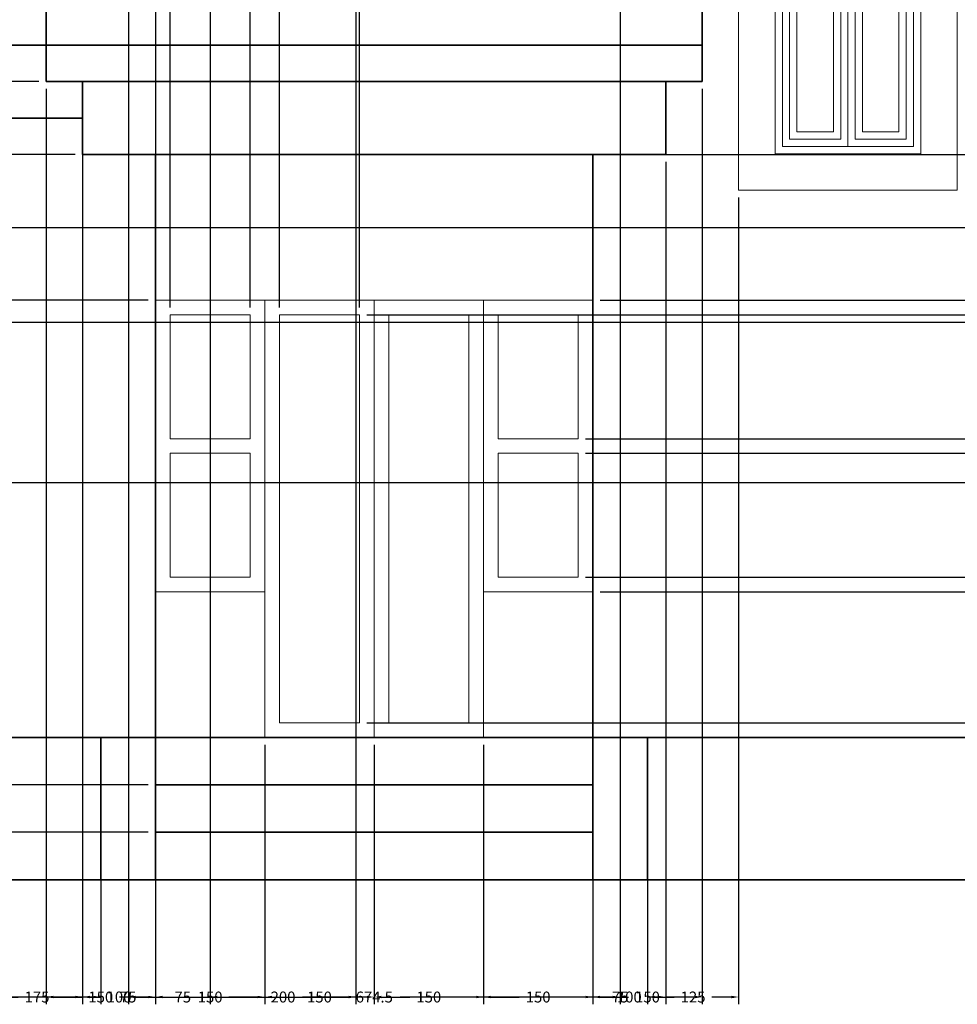
# Model space of a CAD drawing. Units: millimetres. Extents: x 937 to 4561, y 2711 to 5748.
# Tile 5 of 8: x 2543 to 3829, y 2711 to 4062. Entities that reach past the tile are written whole.
import ezdxf

# ---------------------------------------------------------------- set-up
doc = ezdxf.new("R2010")
doc.units = ezdxf.units.MM
doc.header["$MEASUREMENT"] = 0
for name, color, linetype, lineweight in [('A-ANNO-DIMS', 2, 'Continuous', 18), ('A-DOOR', 3, 'Continuous', 18), ('A-ELEV', 7, 'Continuous', 35), ('A-GLAZ', 4, 'Continuous', 18)]:
    doc.layers.add(name, color=color, linetype=linetype, lineweight=lineweight)
doc.styles.get("Standard").update_dxf_attribs({"font": 'arial.ttf'})
doc.dimstyles.get("Standard").update_dxf_attribs({"dimtxt": 15, "dimasz": 10, "dimexe": 10, "dimexo": 10, "dimgap": 10, "dimtad": 0, "dimtih": 1, "dimtoh": 1, "dimdec": 0, "dimzin": 0, "dimdsep": 46, "dimtxsty": 'Standard', "dimcen": 5, "dimadec": 0, "dimazin": 0, "dimtfac": 1, "dimtdec": 0, "dimtofl": 0, "dimtmove": 0, "dimatfit": 3, "dimfxl": 1, "dimtolj": 1, "dimtzin": 0, "dimarcsym": 0})

# ---------------------------------------------------------------- blocks, each defined once
blk = doc.blocks.new('WIN-SIDE')
for p, q in [((3529.5, 5026.9), (3529.5, 4626.9)), ((3579.5, 5026.9), (3779.5, 5026.9)), ((3579.5, 4676.9), (3579.5, 5026.9)), ((3779.5, 5026.9), (3779.5, 4676.9)), ((3829.5, 4626.9), (3829.5, 5026.9)), ((3779.5, 4676.9), (3579.5, 4676.9)), ((3529.5, 4626.9), (3829.5, 4626.9))]:
    blk.add_line(p, q)
for points in [[(3589.5, 5016.9), (3679.5, 5016.9), (3679.5, 4926.9), (3589.5, 4926.9)], [(3679.5, 5016.9), (3769.5, 5016.9), (3769.5, 4926.9), (3679.5, 4926.9)], [(3599.5, 5006.9), (3669.5, 5006.9), (3669.5, 4936.9), (3599.5, 4936.9)], [(3689.5, 5006.9), (3759.5, 5006.9), (3759.5, 4936.9), (3689.5, 4936.9)], [(3609.5, 4996.9), (3659.5, 4996.9), (3659.5, 4946.9), (3609.5, 4946.9)], [(3699.5, 4996.9), (3749.5, 4996.9), (3749.5, 4946.9), (3699.5, 4946.9)], [(3589.5, 4916.9), (3679.5, 4916.9), (3679.5, 4686.9), (3589.5, 4686.9)], [(3599.5, 4906.9), (3669.5, 4906.9), (3669.5, 4696.9), (3599.5, 4696.9)], [(3679.5, 4916.9), (3769.5, 4916.9), (3769.5, 4686.9), (3679.5, 4686.9)], [(3689.5, 4906.9), (3759.5, 4906.9), (3759.5, 4696.9), (3689.5, 4696.9)], [(3609.5, 4896.9), (3659.5, 4896.9), (3659.5, 4706.9), (3609.5, 4706.9)], [(3699.5, 4896.9), (3749.5, 4896.9), (3749.5, 4706.9), (3699.5, 4706.9)]]:
    blk.add_lwpolyline(points, close=True)
blk = doc.blocks.new('*D6')
at = {"layer": 'A-ANNO-DIMS', "color": 0, "lineweight": -2, "transparency": 16777216}
for p, q in [((2479.5, 3066.9), (2479.5, 2710.9)), ((2654.5, 3066.9), (2654.5, 2710.9)), ((2489.5, 2720.9), (2541.1, 2720.9)), ((2644.5, 2720.9), (2592.9, 2720.9))]:
    blk.add_line(p, q, dxfattribs=at)
at = {"layer": 'A-ANNO-DIMS', "color": 0, "transparency": 16777216}
for points in [[(2489.5, 2722.6), (2489.5, 2719.2), (2479.5, 2720.9)], [(2644.5, 2722.6), (2644.5, 2719.2), (2654.5, 2720.9)]]:
    blk.add_solid(points, dxfattribs=at)
at = {"layer": 'Defpoints', "color": 0, "transparency": 16777216}
for p in [(2479.5, 3076.9), (2654.5, 3076.9), (2654.5, 2720.9)]:
    blk.add_point(p, dxfattribs=at)
at = {"layer": 'A-ANNO-DIMS', "color": 0, "transparency": 16777216, "insert": (2567, 2720.9), "char_height": 15, "attachment_point": 5}
blk.add_mtext('\\A1;175', dxfattribs=at)
blk = doc.blocks.new('*D7')
at = {"layer": 'A-ANNO-DIMS', "color": 0, "lineweight": -2, "transparency": 16777216}
for p, q in [((2654.5, 3066.9), (2654.5, 2710.9)), ((2729.5, 3066.9), (2729.5, 2710.9)), ((2644.5, 2720.9), (2634.5, 2720.9)), ((2739.5, 2720.9), (2749.5, 2720.9))]:
    blk.add_line(p, q, dxfattribs=at)
at = {"layer": 'A-ANNO-DIMS', "color": 0, "transparency": 16777216}
for points in [[(2644.5, 2722.6), (2644.5, 2719.2), (2654.5, 2720.9)], [(2739.5, 2722.6), (2739.5, 2719.2), (2729.5, 2720.9)]]:
    blk.add_solid(points, dxfattribs=at)
at = {"layer": 'Defpoints', "color": 0, "transparency": 16777216}
for p in [(2654.5, 3076.9), (2729.5, 3076.9), (2729.5, 2720.9)]:
    blk.add_point(p, dxfattribs=at)
at = {"layer": 'A-ANNO-DIMS', "color": 0, "transparency": 16777216, "insert": (2692, 2720.9), "char_height": 15, "attachment_point": 5}
blk.add_mtext('\\A1;75', dxfattribs=at)
blk = doc.blocks.new('*D8')
at = {"layer": 'A-ANNO-DIMS', "color": 0, "lineweight": -2, "transparency": 16777216}
for p, q in [((2729.5, 3066.9), (2729.5, 2710.9)), ((2879.5, 3066.9), (2879.5, 2710.9)), ((2739.5, 2720.9), (2778.6, 2720.9)), ((2869.5, 2720.9), (2830.3, 2720.9))]:
    blk.add_line(p, q, dxfattribs=at)
at = {"layer": 'A-ANNO-DIMS', "color": 0, "transparency": 16777216}
for points in [[(2739.5, 2722.6), (2739.5, 2719.2), (2729.5, 2720.9)], [(2869.5, 2722.6), (2869.5, 2719.2), (2879.5, 2720.9)]]:
    blk.add_solid(points, dxfattribs=at)
at = {"layer": 'Defpoints', "color": 0, "transparency": 16777216}
for p in [(2729.5, 3076.9), (2879.5, 3076.9), (2879.5, 2720.9)]:
    blk.add_point(p, dxfattribs=at)
at = {"layer": 'A-ANNO-DIMS', "color": 0, "transparency": 16777216, "insert": (2804.5, 2720.9), "char_height": 15, "attachment_point": 5}
blk.add_mtext('\\A1;150', dxfattribs=at)
blk = doc.blocks.new('*D9')
at = {"layer": 'A-ANNO-DIMS', "color": 0, "lineweight": -2, "transparency": 16777216}
for p, q in [((2879.5, 3066.9), (2879.5, 2710.9)), ((3029.5, 3066.9), (3029.5, 2710.9)), ((2889.5, 2720.9), (2928.6, 2720.9)), ((3019.5, 2720.9), (2980.3, 2720.9))]:
    blk.add_line(p, q, dxfattribs=at)
at = {"layer": 'A-ANNO-DIMS', "color": 0, "transparency": 16777216}
for points in [[(2889.5, 2722.6), (2889.5, 2719.2), (2879.5, 2720.9)], [(3019.5, 2722.6), (3019.5, 2719.2), (3029.5, 2720.9)]]:
    blk.add_solid(points, dxfattribs=at)
at = {"layer": 'Defpoints', "color": 0, "transparency": 16777216}
for p in [(2879.5, 3076.9), (3029.5, 3076.9), (3029.5, 2720.9)]:
    blk.add_point(p, dxfattribs=at)
at = {"layer": 'A-ANNO-DIMS', "color": 0, "transparency": 16777216, "insert": (2954.5, 2720.9), "char_height": 15, "attachment_point": 5}
blk.add_mtext('\\A1;150', dxfattribs=at)
blk = doc.blocks.new('*D10')
at = {"layer": 'A-ANNO-DIMS', "color": 0, "lineweight": -2, "transparency": 16777216}
for p, q in [((3029.5, 3066.9), (3029.5, 2710.9)), ((3179.5, 3066.9), (3179.5, 2710.9)), ((3039.5, 2720.9), (3078.6, 2720.9)), ((3169.5, 2720.9), (3130.3, 2720.9))]:
    blk.add_line(p, q, dxfattribs=at)
at = {"layer": 'A-ANNO-DIMS', "color": 0, "transparency": 16777216}
for points in [[(3039.5, 2722.6), (3039.5, 2719.2), (3029.5, 2720.9)], [(3169.5, 2722.6), (3169.5, 2719.2), (3179.5, 2720.9)]]:
    blk.add_solid(points, dxfattribs=at)
at = {"layer": 'Defpoints', "color": 0, "transparency": 16777216}
for p in [(3029.5, 3076.9), (3179.5, 3076.9), (3179.5, 2720.9)]:
    blk.add_point(p, dxfattribs=at)
at = {"layer": 'A-ANNO-DIMS', "color": 0, "transparency": 16777216, "insert": (3104.5, 2720.9), "char_height": 15, "attachment_point": 5}
blk.add_mtext('\\A1;150', dxfattribs=at)
blk = doc.blocks.new('*D11')
at = {"layer": 'A-ANNO-DIMS', "color": 0, "lineweight": -2, "transparency": 16777216}
for p, q in [((3179.5, 3066.9), (3179.5, 2710.9)), ((3329.5, 3066.9), (3329.5, 2710.9)), ((3189.5, 2720.9), (3228.6, 2720.9)), ((3319.5, 2720.9), (3280.3, 2720.9))]:
    blk.add_line(p, q, dxfattribs=at)
at = {"layer": 'A-ANNO-DIMS', "color": 0, "transparency": 16777216}
for points in [[(3189.5, 2722.6), (3189.5, 2719.2), (3179.5, 2720.9)], [(3319.5, 2722.6), (3319.5, 2719.2), (3329.5, 2720.9)]]:
    blk.add_solid(points, dxfattribs=at)
at = {"layer": 'Defpoints', "color": 0, "transparency": 16777216}
for p in [(3179.5, 3076.9), (3329.5, 3076.9), (3329.5, 2720.9)]:
    blk.add_point(p, dxfattribs=at)
at = {"layer": 'A-ANNO-DIMS', "color": 0, "transparency": 16777216, "insert": (3254.5, 2720.9), "char_height": 15, "attachment_point": 5}
blk.add_mtext('\\A1;150', dxfattribs=at)
blk = doc.blocks.new('*D12')
at = {"layer": 'A-ANNO-DIMS', "color": 0, "lineweight": -2, "transparency": 16777216}
for p, q in [((3329.5, 3066.9), (3329.5, 2710.9)), ((3404.5, 3066.9), (3404.5, 2710.9)), ((3319.5, 2720.9), (3309.5, 2720.9)), ((3414.5, 2720.9), (3424.5, 2720.9))]:
    blk.add_line(p, q, dxfattribs=at)
at = {"layer": 'A-ANNO-DIMS', "color": 0, "transparency": 16777216}
for points in [[(3319.5, 2722.6), (3319.5, 2719.2), (3329.5, 2720.9)], [(3414.5, 2722.6), (3414.5, 2719.2), (3404.5, 2720.9)]]:
    blk.add_solid(points, dxfattribs=at)
at = {"layer": 'Defpoints', "color": 0, "transparency": 16777216}
for p in [(3329.5, 3076.9), (3404.5, 3076.9), (3404.5, 2720.9)]:
    blk.add_point(p, dxfattribs=at)
at = {"layer": 'A-ANNO-DIMS', "color": 0, "transparency": 16777216, "insert": (3367, 2720.9), "char_height": 15, "attachment_point": 5}
blk.add_mtext('\\A1;75', dxfattribs=at)
blk = doc.blocks.new('*D13')
at = {"layer": 'A-ANNO-DIMS', "color": 0, "lineweight": -2, "transparency": 16777216}
for p, q in [((3529.5, 3817.9), (3529.5, 2710.9)), ((3404.5, 3066.9), (3404.5, 2710.9)), ((3414.5, 2720.9), (3441.1, 2720.9)), ((3519.5, 2720.9), (3492.9, 2720.9))]:
    blk.add_line(p, q, dxfattribs=at)
at = {"layer": 'A-ANNO-DIMS', "color": 0, "transparency": 16777216}
for points in [[(3414.5, 2722.6), (3414.5, 2719.2), (3404.5, 2720.9)], [(3519.5, 2722.6), (3519.5, 2719.2), (3529.5, 2720.9)]]:
    blk.add_solid(points, dxfattribs=at)
at = {"layer": 'Defpoints', "color": 0, "transparency": 16777216}
for p in [(3529.5, 3827.9), (3404.5, 3076.9), (3529.5, 2720.9)]:
    blk.add_point(p, dxfattribs=at)
at = {"layer": 'A-ANNO-DIMS', "color": 0, "transparency": 16777216, "insert": (3467, 2720.9), "char_height": 15, "attachment_point": 5}
blk.add_mtext('\\A1;125', dxfattribs=at)
blk = doc.blocks.new('*D24')
at = {"layer": 'A-ANNO-DIMS', "color": 0, "lineweight": -2, "transparency": 16777216}
for p, q in [((2692.4, 4642.9), (2692.4, 2710.9)), ((3366.9, 4642.9), (3366.9, 2710.9)), ((2702.4, 2720.9), (2994.3, 2720.9)), ((3356.9, 2720.9), (3065.1, 2720.9))]:
    blk.add_line(p, q, dxfattribs=at)
at = {"layer": 'A-ANNO-DIMS', "color": 0, "transparency": 16777216}
for points in [[(2702.4, 2722.6), (2702.4, 2719.2), (2692.4, 2720.9)], [(3356.9, 2722.6), (3356.9, 2719.2), (3366.9, 2720.9)]]:
    blk.add_solid(points, dxfattribs=at)
at = {"layer": 'Defpoints', "color": 0, "transparency": 16777216}
for p in [(2692.4, 4652.9), (3366.9, 4652.9), (3366.9, 2720.9)]:
    blk.add_point(p, dxfattribs=at)
at = {"layer": 'A-ANNO-DIMS', "color": 0, "transparency": 16777216, "insert": (3029.7, 2720.9), "char_height": 15, "attachment_point": 5}
blk.add_mtext('\\A1;674.5', dxfattribs=at)
blk = doc.blocks.new('*D44')
at = {"layer": 'A-ANNO-DIMS', "color": 0, "lineweight": -2, "transparency": 16777216}
for p, q in [((1379.5, 3916.9), (1379.5, 2710.9)), ((2629.5, 3916.9), (2629.5, 2710.9)), ((1389.5, 2720.9), (1972.8, 2720.9)), ((2619.5, 2720.9), (2036.2, 2720.9))]:
    blk.add_line(p, q, dxfattribs=at)
at = {"layer": 'A-ANNO-DIMS', "color": 0, "transparency": 16777216}
for points in [[(1389.5, 2722.6), (1389.5, 2719.2), (1379.5, 2720.9)], [(2619.5, 2722.6), (2619.5, 2719.2), (2629.5, 2720.9)]]:
    blk.add_solid(points, dxfattribs=at)
at = {"layer": 'Defpoints', "color": 0, "transparency": 16777216}
for p in [(1379.5, 3926.9), (2629.5, 3926.9), (2629.5, 2720.9)]:
    blk.add_point(p, dxfattribs=at)
at = {"layer": 'A-ANNO-DIMS', "color": 0, "transparency": 16777216, "insert": (2004.5, 2720.9), "char_height": 15, "attachment_point": 5}
blk.add_mtext('\\A1;1250', dxfattribs=at)
blk = doc.blocks.new('*D45')
at = {"layer": 'A-ANNO-DIMS', "color": 0, "lineweight": -2, "transparency": 16777216}
for p, q in [((2579.5, 3966.9), (2579.5, 2710.9)), ((2729.5, 3866.9), (2729.5, 2710.9)), ((2589.5, 2720.9), (2628.6, 2720.9)), ((2719.5, 2720.9), (2680.3, 2720.9))]:
    blk.add_line(p, q, dxfattribs=at)
at = {"layer": 'A-ANNO-DIMS', "color": 0, "transparency": 16777216}
for points in [[(2589.5, 2722.6), (2589.5, 2719.2), (2579.5, 2720.9)], [(2719.5, 2722.6), (2719.5, 2719.2), (2729.5, 2720.9)]]:
    blk.add_solid(points, dxfattribs=at)
at = {"layer": 'Defpoints', "color": 0, "transparency": 16777216}
for p in [(2579.5, 3976.9), (2729.5, 3876.9), (2729.5, 2720.9)]:
    blk.add_point(p, dxfattribs=at)
at = {"layer": 'A-ANNO-DIMS', "color": 0, "transparency": 16777216, "insert": (2654.5, 2720.9), "char_height": 15, "attachment_point": 5}
blk.add_mtext('\\A1;150', dxfattribs=at)
blk = doc.blocks.new('*D46')
at = {"layer": 'A-ANNO-DIMS', "color": 0, "lineweight": -2, "transparency": 16777216}
for p, q in [((2629.5, 3866.9), (2629.5, 2710.9)), ((2729.5, 3866.9), (2729.5, 2710.9)), ((2639.5, 2720.9), (2653.6, 2720.9)), ((2719.5, 2720.9), (2705.3, 2720.9))]:
    blk.add_line(p, q, dxfattribs=at)
at = {"layer": 'A-ANNO-DIMS', "color": 0, "transparency": 16777216}
for points in [[(2639.5, 2722.6), (2639.5, 2719.2), (2629.5, 2720.9)], [(2719.5, 2722.6), (2719.5, 2719.2), (2729.5, 2720.9)]]:
    blk.add_solid(points, dxfattribs=at)
at = {"layer": 'Defpoints', "color": 0, "transparency": 16777216}
for p in [(2629.5, 3876.9), (2729.5, 3876.9), (2729.5, 2720.9)]:
    blk.add_point(p, dxfattribs=at)
at = {"layer": 'A-ANNO-DIMS', "color": 0, "transparency": 16777216, "insert": (2679.5, 2720.9), "char_height": 15, "attachment_point": 5}
blk.add_mtext('\\A1;100', dxfattribs=at)
blk = doc.blocks.new('*D47')
at = {"layer": 'A-ANNO-DIMS', "color": 0, "lineweight": -2, "transparency": 16777216}
for p, q in [((3329.5, 3866.9), (3329.5, 2710.9)), ((3429.5, 3866.9), (3429.5, 2710.9)), ((3339.5, 2720.9), (3353.6, 2720.9)), ((3419.5, 2720.9), (3405.3, 2720.9))]:
    blk.add_line(p, q, dxfattribs=at)
at = {"layer": 'A-ANNO-DIMS', "color": 0, "transparency": 16777216}
for points in [[(3339.5, 2722.6), (3339.5, 2719.2), (3329.5, 2720.9)], [(3419.5, 2722.6), (3419.5, 2719.2), (3429.5, 2720.9)]]:
    blk.add_solid(points, dxfattribs=at)
at = {"layer": 'Defpoints', "color": 0, "transparency": 16777216}
for p in [(3329.5, 3876.9), (3429.5, 3876.9), (3429.5, 2720.9)]:
    blk.add_point(p, dxfattribs=at)
at = {"layer": 'A-ANNO-DIMS', "color": 0, "transparency": 16777216, "insert": (3379.5, 2720.9), "char_height": 15, "attachment_point": 5}
blk.add_mtext('\\A1;100', dxfattribs=at)
blk = doc.blocks.new('*D48')
at = {"layer": 'A-ANNO-DIMS', "color": 0, "lineweight": -2, "transparency": 16777216}
for p, q in [((3479.5, 3966.9), (3479.5, 2710.9)), ((3329.5, 3866.9), (3329.5, 2710.9)), ((3339.5, 2720.9), (3378.6, 2720.9)), ((3469.5, 2720.9), (3430.3, 2720.9))]:
    blk.add_line(p, q, dxfattribs=at)
at = {"layer": 'A-ANNO-DIMS', "color": 0, "transparency": 16777216}
for points in [[(3339.5, 2722.6), (3339.5, 2719.2), (3329.5, 2720.9)], [(3469.5, 2722.6), (3469.5, 2719.2), (3479.5, 2720.9)]]:
    blk.add_solid(points, dxfattribs=at)
at = {"layer": 'Defpoints', "color": 0, "transparency": 16777216}
for p in [(3479.5, 3976.9), (3329.5, 3876.9), (3479.5, 2720.9)]:
    blk.add_point(p, dxfattribs=at)
at = {"layer": 'A-ANNO-DIMS', "color": 0, "transparency": 16777216, "insert": (3404.5, 2720.9), "char_height": 15, "attachment_point": 5}
blk.add_mtext('\\A1;150', dxfattribs=at)
blk = doc.blocks.new('*D49')
at = {"layer": 'A-ANNO-DIMS', "color": 0, "lineweight": -2, "transparency": 16777216}
for p, q in [((2729.5, 4242.9), (2729.5, 2710.9)), ((2804.5, 4217.9), (2804.5, 2710.9)), ((2719.5, 2720.9), (2709.5, 2720.9)), ((2814.5, 2720.9), (2824.5, 2720.9))]:
    blk.add_line(p, q, dxfattribs=at)
at = {"layer": 'A-ANNO-DIMS', "color": 0, "transparency": 16777216}
for points in [[(2719.5, 2722.6), (2719.5, 2719.2), (2729.5, 2720.9)], [(2814.5, 2722.6), (2814.5, 2719.2), (2804.5, 2720.9)]]:
    blk.add_solid(points, dxfattribs=at)
at = {"layer": 'Defpoints', "color": 0, "transparency": 16777216}
for p in [(2729.5, 4252.9), (2804.5, 4227.9), (2804.5, 2720.9)]:
    blk.add_point(p, dxfattribs=at)
at = {"layer": 'A-ANNO-DIMS', "color": 0, "transparency": 16777216, "insert": (2767, 2720.9), "char_height": 15, "attachment_point": 5}
blk.add_mtext('\\A1;75', dxfattribs=at)
blk = doc.blocks.new('*D50')
at = {"layer": 'A-ANNO-DIMS', "color": 0, "lineweight": -2, "transparency": 16777216}
for p, q in [((2804.5, 4217.9), (2804.5, 2710.9)), ((3004.5, 4217.9), (3004.5, 2710.9)), ((2814.5, 2720.9), (2877.8, 2720.9)), ((2994.5, 2720.9), (2931.2, 2720.9))]:
    blk.add_line(p, q, dxfattribs=at)
at = {"layer": 'A-ANNO-DIMS', "color": 0, "transparency": 16777216}
for points in [[(2814.5, 2722.6), (2814.5, 2719.2), (2804.5, 2720.9)], [(2994.5, 2722.6), (2994.5, 2719.2), (3004.5, 2720.9)]]:
    blk.add_solid(points, dxfattribs=at)
at = {"layer": 'Defpoints', "color": 0, "transparency": 16777216}
for p in [(2804.5, 4227.9), (3004.5, 4227.9), (3004.5, 2720.9)]:
    blk.add_point(p, dxfattribs=at)
at = {"layer": 'A-ANNO-DIMS', "color": 0, "transparency": 16777216, "insert": (2904.5, 2720.9), "char_height": 15, "attachment_point": 5}
blk.add_mtext('\\A1;200', dxfattribs=at)
blk = doc.blocks.new('*D53')
at = {"layer": 'A-ANNO-DIMS', "color": 0, "lineweight": -2, "transparency": 16777216}
for p, q in [((2749.5, 3666.9), (2749.5, 5747.9)), ((2859.5, 3666.9), (2859.5, 5747.9)), ((2759.5, 5737.9), (2778.6, 5737.9)), ((2849.5, 5737.9), (2830.3, 5737.9))]:
    blk.add_line(p, q, dxfattribs=at)
at = {"layer": 'A-ANNO-DIMS', "color": 0, "transparency": 16777216}
for points in [[(2759.5, 5739.6), (2759.5, 5736.2), (2749.5, 5737.9)], [(2849.5, 5739.6), (2849.5, 5736.2), (2859.5, 5737.9)]]:
    blk.add_solid(points, dxfattribs=at)
at = {"layer": 'Defpoints', "color": 0, "transparency": 16777216}
for p in [(2859.5, 5737.9), (2749.5, 3656.9), (2859.5, 3656.9)]:
    blk.add_point(p, dxfattribs=at)
at = {"layer": 'A-ANNO-DIMS', "color": 0, "transparency": 16777216, "insert": (2804.5, 5737.9), "char_height": 15, "attachment_point": 5}
blk.add_mtext('\\A1;110', dxfattribs=at)
blk = doc.blocks.new('*D54')
at = {"layer": 'A-ANNO-DIMS', "color": 0, "lineweight": -2, "transparency": 16777216}
for p, q in [((2899.5, 3666.9), (2899.5, 5747.9)), ((3009.5, 3666.9), (3009.5, 5747.9)), ((2909.5, 5737.9), (2928.6, 5737.9)), ((2999.5, 5737.9), (2980.3, 5737.9))]:
    blk.add_line(p, q, dxfattribs=at)
at = {"layer": 'A-ANNO-DIMS', "color": 0, "transparency": 16777216}
for points in [[(2909.5, 5739.6), (2909.5, 5736.2), (2899.5, 5737.9)], [(2999.5, 5739.6), (2999.5, 5736.2), (3009.5, 5737.9)]]:
    blk.add_solid(points, dxfattribs=at)
at = {"layer": 'Defpoints', "color": 0, "transparency": 16777216}
for p in [(3009.5, 5737.9), (2899.5, 3656.9), (3009.5, 3656.9)]:
    blk.add_point(p, dxfattribs=at)
at = {"layer": 'A-ANNO-DIMS', "color": 0, "transparency": 16777216, "insert": (2954.5, 5737.9), "char_height": 15, "attachment_point": 5}
blk.add_mtext('\\A1;110', dxfattribs=at)
blk = doc.blocks.new('*D72')
at = {"layer": 'A-ANNO-DIMS', "color": 0, "lineweight": -2, "transparency": 16777216}
for p, q in [((1764.5, 3646.9), (4500.5, 3646.9)), ((4490.5, 3636.9), (4490.5, 3554.6)), ((4490.5, 3436.9), (4490.5, 3519.2)), ((1764.5, 3426.9), (4500.5, 3426.9))]:
    blk.add_line(p, q, dxfattribs=at)
at = {"layer": 'A-ANNO-DIMS', "color": 0, "transparency": 16777216}
for points in [[(4488.8, 3636.9), (4492.2, 3636.9), (4490.5, 3646.9)], [(4488.8, 3436.9), (4492.2, 3436.9), (4490.5, 3426.9)]]:
    blk.add_solid(points, dxfattribs=at)
at = {"layer": 'Defpoints', "color": 0, "transparency": 16777216}
for p in [(1754.5, 3646.9), (4490.5, 3646.9), (1754.5, 3426.9)]:
    blk.add_point(p, dxfattribs=at)
at = {"layer": 'A-ANNO-DIMS', "color": 0, "transparency": 16777216, "insert": (4490.5, 3536.9), "char_height": 15, "attachment_point": 5}
blk.add_mtext('\\A1;220', dxfattribs=at)
blk = doc.blocks.new('*D73')
at = {"layer": 'A-ANNO-DIMS', "color": 0, "lineweight": -2, "transparency": 16777216}
for p, q in [((1764.5, 3776.9), (4500.5, 3776.9)), ((4490.5, 3766.9), (4490.5, 3729.6)), ((4490.5, 3656.9), (4490.5, 3694.2)), ((1764.5, 3646.9), (4500.5, 3646.9))]:
    blk.add_line(p, q, dxfattribs=at)
at = {"layer": 'A-ANNO-DIMS', "color": 0, "transparency": 16777216}
for points in [[(4488.8, 3766.9), (4492.2, 3766.9), (4490.5, 3776.9)], [(4488.8, 3656.9), (4492.2, 3656.9), (4490.5, 3646.9)]]:
    blk.add_solid(points, dxfattribs=at)
at = {"layer": 'Defpoints', "color": 0, "transparency": 16777216}
for p in [(1754.5, 3776.9), (4490.5, 3776.9), (1754.5, 3646.9)]:
    blk.add_point(p, dxfattribs=at)
at = {"layer": 'A-ANNO-DIMS', "color": 0, "transparency": 16777216, "insert": (4490.5, 3711.9), "char_height": 15, "attachment_point": 5}
blk.add_mtext('\\A1;130', dxfattribs=at)
blk = doc.blocks.new('*D82')
at = {"layer": 'A-ANNO-DIMS', "color": 0, "lineweight": -2, "transparency": 16777216}
for p, q in [((2719.5, 3676.9), (958.5, 3676.9)), ((968.5, 3666.9), (968.5, 3394.6)), ((968.5, 3086.9), (968.5, 3359.2)), ((2719.5, 3076.9), (958.5, 3076.9))]:
    blk.add_line(p, q, dxfattribs=at)
at = {"layer": 'A-ANNO-DIMS', "color": 0, "transparency": 16777216}
for points in [[(966.8, 3666.9), (970.2, 3666.9), (968.5, 3676.9)], [(966.8, 3086.9), (970.2, 3086.9), (968.5, 3076.9)]]:
    blk.add_solid(points, dxfattribs=at)
at = {"layer": 'Defpoints', "color": 0, "transparency": 16777216}
for p in [(968.5, 3676.9), (2729.5, 3676.9), (2729.5, 3076.9)]:
    blk.add_point(p, dxfattribs=at)
at = {"layer": 'A-ANNO-DIMS', "color": 0, "transparency": 16777216, "insert": (968.5, 3376.9), "char_height": 15, "attachment_point": 5}
blk.add_mtext('\\A1;600', dxfattribs=at)
blk = doc.blocks.new('*D83')
at = {"layer": 'A-ANNO-DIMS', "color": 0, "lineweight": -2, "transparency": 16777216}
for p, q in [((2619.5, 3876.9), (958.5, 3876.9)), ((968.5, 3866.9), (968.5, 3794.6)), ((968.5, 3686.9), (968.5, 3759.2)), ((2719.5, 3676.9), (958.5, 3676.9))]:
    blk.add_line(p, q, dxfattribs=at)
at = {"layer": 'A-ANNO-DIMS', "color": 0, "transparency": 16777216}
for points in [[(966.8, 3866.9), (970.2, 3866.9), (968.5, 3876.9)], [(966.8, 3686.9), (970.2, 3686.9), (968.5, 3676.9)]]:
    blk.add_solid(points, dxfattribs=at)
at = {"layer": 'Defpoints', "color": 0, "transparency": 16777216}
for p in [(968.5, 3876.9), (2629.5, 3876.9), (2729.5, 3676.9)]:
    blk.add_point(p, dxfattribs=at)
at = {"layer": 'A-ANNO-DIMS', "color": 0, "transparency": 16777216, "insert": (968.5, 3776.9), "char_height": 15, "attachment_point": 5}
blk.add_mtext('\\A1;200', dxfattribs=at)
blk = doc.blocks.new('*D84')
at = {"layer": 'A-ANNO-DIMS', "color": 0, "lineweight": -2, "transparency": 16777216}
for p, q in [((2569.5, 3976.9), (958.5, 3976.9)), ((968.5, 3966.9), (968.5, 3944.6)), ((968.5, 3886.9), (968.5, 3909.2)), ((2619.5, 3876.9), (958.5, 3876.9))]:
    blk.add_line(p, q, dxfattribs=at)
at = {"layer": 'A-ANNO-DIMS', "color": 0, "transparency": 16777216}
for points in [[(966.8, 3966.9), (970.2, 3966.9), (968.5, 3976.9)], [(966.8, 3886.9), (970.2, 3886.9), (968.5, 3876.9)]]:
    blk.add_solid(points, dxfattribs=at)
at = {"layer": 'Defpoints', "color": 0, "transparency": 16777216}
for p in [(968.5, 3976.9), (2579.5, 3976.9), (2629.5, 3876.9)]:
    blk.add_point(p, dxfattribs=at)
at = {"layer": 'A-ANNO-DIMS', "color": 0, "transparency": 16777216, "insert": (968.5, 3926.9), "char_height": 15, "attachment_point": 5}
blk.add_mtext('\\A1;100', dxfattribs=at)
blk = doc.blocks.new('*D85')
at = {"layer": 'A-ANNO-DIMS', "color": 0, "lineweight": -2, "transparency": 16777216}
for p, q in [((2569.5, 4026.9), (958.5, 4026.9)), ((968.5, 4026.9), (968.5, 4036.9)), ((968.5, 4036.9), (978.5, 4036.9)), ((968.5, 3986.9), (968.5, 4016.9)), ((2569.5, 3976.9), (958.5, 3976.9))]:
    blk.add_line(p, q, dxfattribs=at)
at = {"layer": 'A-ANNO-DIMS', "color": 0, "transparency": 16777216}
for points in [[(966.8, 4016.9), (970.2, 4016.9), (968.5, 4026.9)], [(966.8, 3986.9), (970.2, 3986.9), (968.5, 3976.9)]]:
    blk.add_solid(points, dxfattribs=at)
at = {"layer": 'Defpoints', "color": 0, "transparency": 16777216}
for p in [(968.5, 4026.9), (2579.5, 4026.9), (2579.5, 3976.9)]:
    blk.add_point(p, dxfattribs=at)
at = {"layer": 'A-ANNO-DIMS', "color": 0, "transparency": 16777216, "insert": (999.2, 4036.9), "char_height": 15, "attachment_point": 5}
blk.add_mtext('\\A1;50', dxfattribs=at)
blk = doc.blocks.new('*D86')
at = {"layer": 'A-ANNO-DIMS', "color": 0, "lineweight": -2, "transparency": 16777216}
for p, q in [((968.5, 4076.9), (968.5, 4086.9)), ((968.5, 4086.9), (978.5, 4086.9)), ((2569.5, 4076.9), (958.5, 4076.9)), ((968.5, 4036.9), (968.5, 4066.9)), ((2569.5, 4026.9), (958.5, 4026.9))]:
    blk.add_line(p, q, dxfattribs=at)
at = {"layer": 'A-ANNO-DIMS', "color": 0, "transparency": 16777216}
for points in [[(966.8, 4066.9), (970.2, 4066.9), (968.5, 4076.9)], [(966.8, 4036.9), (970.2, 4036.9), (968.5, 4026.9)]]:
    blk.add_solid(points, dxfattribs=at)
at = {"layer": 'Defpoints', "color": 0, "transparency": 16777216}
for p in [(968.5, 4076.9), (2579.5, 4076.9), (2579.5, 4026.9)]:
    blk.add_point(p, dxfattribs=at)
at = {"layer": 'A-ANNO-DIMS', "color": 0, "transparency": 16777216, "insert": (999.2, 4086.9), "char_height": 15, "attachment_point": 5}
blk.add_mtext('\\A1;50', dxfattribs=at)
blk = doc.blocks.new('*D94')
at = {"layer": 'A-ANNO-DIMS', "color": 0, "lineweight": -2, "transparency": 16777216}
for p, q in [((3339.5, 3276.9), (4500.5, 3276.9)), ((4490.5, 3266.9), (4490.5, 3194.6)), ((4490.5, 3086.9), (4490.5, 3159.2)), ((3339.5, 3076.9), (4500.5, 3076.9))]:
    blk.add_line(p, q, dxfattribs=at)
at = {"layer": 'A-ANNO-DIMS', "color": 0, "transparency": 16777216}
for points in [[(4488.8, 3266.9), (4492.2, 3266.9), (4490.5, 3276.9)], [(4488.8, 3086.9), (4492.2, 3086.9), (4490.5, 3076.9)]]:
    blk.add_solid(points, dxfattribs=at)
at = {"layer": 'Defpoints', "color": 0, "transparency": 16777216}
for p in [(3329.5, 3276.9), (4490.5, 3276.9), (3329.5, 3076.9)]:
    blk.add_point(p, dxfattribs=at)
at = {"layer": 'A-ANNO-DIMS', "color": 0, "transparency": 16777216, "insert": (4490.5, 3176.9), "char_height": 15, "attachment_point": 5}
blk.add_mtext('\\A1;200', dxfattribs=at)
blk = doc.blocks.new('*D95')
at = {"layer": 'A-ANNO-DIMS', "color": 0, "lineweight": -2, "transparency": 16777216}
for p, q in [((3319.5, 3486.9), (4500.5, 3486.9)), ((4490.5, 3476.9), (4490.5, 3409.6)), ((4490.5, 3306.9), (4490.5, 3374.2)), ((3319.5, 3296.9), (4500.5, 3296.9))]:
    blk.add_line(p, q, dxfattribs=at)
at = {"layer": 'A-ANNO-DIMS', "color": 0, "transparency": 16777216}
for points in [[(4488.8, 3476.9), (4492.2, 3476.9), (4490.5, 3486.9)], [(4488.8, 3306.9), (4492.2, 3306.9), (4490.5, 3296.9)]]:
    blk.add_solid(points, dxfattribs=at)
at = {"layer": 'Defpoints', "color": 0, "transparency": 16777216}
for p in [(3309.5, 3486.9), (4490.5, 3486.9), (3309.5, 3296.9)]:
    blk.add_point(p, dxfattribs=at)
at = {"layer": 'A-ANNO-DIMS', "color": 0, "transparency": 16777216, "insert": (4490.5, 3391.9), "char_height": 15, "attachment_point": 5}
blk.add_mtext('\\A1;190', dxfattribs=at)
blk = doc.blocks.new('*D96')
at = {"layer": 'A-ANNO-DIMS', "color": 0, "lineweight": -2, "transparency": 16777216}
for p, q in [((3319.5, 3656.9), (4500.5, 3656.9)), ((4490.5, 3646.9), (4490.5, 3579.6)), ((4490.5, 3476.9), (4490.5, 3544.2)), ((3319.5, 3466.9), (4500.5, 3466.9))]:
    blk.add_line(p, q, dxfattribs=at)
at = {"layer": 'A-ANNO-DIMS', "color": 0, "transparency": 16777216}
for points in [[(4488.8, 3646.9), (4492.2, 3646.9), (4490.5, 3656.9)], [(4488.8, 3476.9), (4492.2, 3476.9), (4490.5, 3466.9)]]:
    blk.add_solid(points, dxfattribs=at)
at = {"layer": 'Defpoints', "color": 0, "transparency": 16777216}
for p in [(3309.5, 3656.9), (4490.5, 3656.9), (3309.5, 3466.9)]:
    blk.add_point(p, dxfattribs=at)
at = {"layer": 'A-ANNO-DIMS', "color": 0, "transparency": 16777216, "insert": (4490.5, 3561.9), "char_height": 15, "attachment_point": 5}
blk.add_mtext('\\A1;190', dxfattribs=at)
blk = doc.blocks.new('*D97')
at = {"layer": 'A-ANNO-DIMS', "color": 0, "lineweight": -2, "transparency": 16777216}
for p, q in [((3339.5, 3876.9), (4500.5, 3876.9)), ((4490.5, 3866.9), (4490.5, 3794.6)), ((4490.5, 3686.9), (4490.5, 3759.2)), ((3339.5, 3676.9), (4500.5, 3676.9))]:
    blk.add_line(p, q, dxfattribs=at)
at = {"layer": 'A-ANNO-DIMS', "color": 0, "transparency": 16777216}
for points in [[(4488.8, 3866.9), (4492.2, 3866.9), (4490.5, 3876.9)], [(4488.8, 3686.9), (4492.2, 3686.9), (4490.5, 3676.9)]]:
    blk.add_solid(points, dxfattribs=at)
at = {"layer": 'Defpoints', "color": 0, "transparency": 16777216}
for p in [(3329.5, 3876.9), (4490.5, 3876.9), (3329.5, 3676.9)]:
    blk.add_point(p, dxfattribs=at)
at = {"layer": 'A-ANNO-DIMS', "color": 0, "transparency": 16777216, "insert": (4490.5, 3776.9), "char_height": 15, "attachment_point": 5}
blk.add_mtext('\\A1;200', dxfattribs=at)
blk = doc.blocks.new('*D98')
at = {"layer": 'A-ANNO-DIMS', "color": 0, "lineweight": -2, "transparency": 16777216}
for p, q in [((3019.5, 3656.9), (4500.5, 3656.9)), ((4490.5, 3646.9), (4490.5, 3394.6)), ((4490.5, 3106.9), (4490.5, 3359.2)), ((3019.5, 3096.9), (4500.5, 3096.9))]:
    blk.add_line(p, q, dxfattribs=at)
at = {"layer": 'A-ANNO-DIMS', "color": 0, "transparency": 16777216}
for points in [[(4488.8, 3646.9), (4492.2, 3646.9), (4490.5, 3656.9)], [(4488.8, 3106.9), (4492.2, 3106.9), (4490.5, 3096.9)]]:
    blk.add_solid(points, dxfattribs=at)
at = {"layer": 'Defpoints', "color": 0, "transparency": 16777216}
for p in [(3009.5, 3656.9), (4490.5, 3656.9), (3009.5, 3096.9)]:
    blk.add_point(p, dxfattribs=at)
at = {"layer": 'A-ANNO-DIMS', "color": 0, "transparency": 16777216, "insert": (4490.5, 3376.9), "char_height": 15, "attachment_point": 5}
blk.add_mtext('\\A1;560', dxfattribs=at)
blk = doc.blocks.new('*D99')
at = {"layer": 'A-ANNO-DIMS', "color": 0, "lineweight": -2, "transparency": 16777216}
for p, q in [((2719.5, 2946.9), (958.5, 2946.9)), ((968.5, 2946.9), (968.5, 2956.9)), ((968.5, 2956.9), (978.5, 2956.9)), ((968.5, 2891.9), (968.5, 2936.9)), ((2644.5, 2881.9), (958.5, 2881.9))]:
    blk.add_line(p, q, dxfattribs=at)
at = {"layer": 'A-ANNO-DIMS', "color": 0, "transparency": 16777216}
for points in [[(966.8, 2936.9), (970.2, 2936.9), (968.5, 2946.9)], [(966.8, 2891.9), (970.2, 2891.9), (968.5, 2881.9)]]:
    blk.add_solid(points, dxfattribs=at)
at = {"layer": 'Defpoints', "color": 0, "transparency": 16777216}
for p in [(968.5, 2946.9), (2729.5, 2946.9), (2654.5, 2881.9)]:
    blk.add_point(p, dxfattribs=at)
at = {"layer": 'A-ANNO-DIMS', "color": 0, "transparency": 16777216, "insert": (999.3, 2956.9), "char_height": 15, "attachment_point": 5}
blk.add_mtext('\\A1;65', dxfattribs=at)
blk = doc.blocks.new('*D100')
at = {"layer": 'A-ANNO-DIMS', "color": 0, "lineweight": -2, "transparency": 16777216}
for p, q in [((968.5, 3011.9), (968.5, 3021.9)), ((968.5, 3021.9), (978.5, 3021.9)), ((2719.5, 3011.9), (958.5, 3011.9)), ((968.5, 2956.9), (968.5, 3001.9)), ((2719.5, 2946.9), (958.5, 2946.9))]:
    blk.add_line(p, q, dxfattribs=at)
at = {"layer": 'A-ANNO-DIMS', "color": 0, "transparency": 16777216}
for points in [[(966.8, 3001.9), (970.2, 3001.9), (968.5, 3011.9)], [(966.8, 2956.9), (970.2, 2956.9), (968.5, 2946.9)]]:
    blk.add_solid(points, dxfattribs=at)
at = {"layer": 'Defpoints', "color": 0, "transparency": 16777216}
for p in [(968.5, 3011.9), (2729.5, 3011.9), (2729.5, 2946.9)]:
    blk.add_point(p, dxfattribs=at)
at = {"layer": 'A-ANNO-DIMS', "color": 0, "transparency": 16777216, "insert": (999.3, 3021.9), "char_height": 15, "attachment_point": 5}
blk.add_mtext('\\A1;65', dxfattribs=at)
blk = doc.blocks.new('*D101')
at = {"layer": 'A-ANNO-DIMS', "color": 0, "lineweight": -2, "transparency": 16777216}
for p, q in [((968.5, 3076.9), (968.5, 3086.9)), ((968.5, 3086.9), (978.5, 3086.9)), ((2644.5, 3076.9), (958.5, 3076.9)), ((968.5, 3021.9), (968.5, 3066.9)), ((2719.5, 3011.9), (958.5, 3011.9))]:
    blk.add_line(p, q, dxfattribs=at)
at = {"layer": 'A-ANNO-DIMS', "color": 0, "transparency": 16777216}
for points in [[(966.8, 3066.9), (970.2, 3066.9), (968.5, 3076.9)], [(966.8, 3021.9), (970.2, 3021.9), (968.5, 3011.9)]]:
    blk.add_solid(points, dxfattribs=at)
at = {"layer": 'Defpoints', "color": 0, "transparency": 16777216}
for p in [(968.5, 3076.9), (2654.5, 3076.9), (2729.5, 3011.9)]:
    blk.add_point(p, dxfattribs=at)
at = {"layer": 'A-ANNO-DIMS', "color": 0, "transparency": 16777216, "insert": (999.3, 3086.9), "char_height": 15, "attachment_point": 5}
blk.add_mtext('\\A1;65', dxfattribs=at)

msp = doc.modelspace()

# ---------------------------------------------------------------- linework, layer by layer
at = {"layer": 'A-DOOR'}
for p, q in [((2879.4852, 3676.9013), (3029.4852, 3676.9013)), ((2879.4852, 3076.9013), (2879.4852, 3676.9013)), ((3029.4852, 3676.9013), (3179.4852, 3676.9013)), ((3029.4852, 3076.9013), (3029.4852, 3676.9013)), ((3029.4852, 3676.9013), (3029.4852, 3076.9013)), ((3179.4852, 3676.9013), (3179.4852, 3076.9013)), ((2899.4852, 3656.9013), (3009.4852, 3656.9013)), ((2899.4852, 3096.9013), (2899.4852, 3656.9013)), ((3009.4852, 3656.9013), (3009.4852, 3096.9013)), ((3049.4852, 3656.9013), (3159.4852, 3656.9013)), ((3049.4852, 3096.9013), (3049.4852, 3656.9013)), ((3159.4852, 3656.9013), (3159.4852, 3096.9013)), ((2749.4852, 3486.9013), (2859.4852, 3486.9013)), ((3199.4852, 3486.9013), (3309.4852, 3486.9013)), ((2749.4852, 3466.9013), (2859.4852, 3466.9013)), ((3199.4852, 3466.9013), (3309.4852, 3466.9013)), ((3009.4852, 3096.9013), (2899.4852, 3096.9013)), ((3159.4852, 3096.9013), (3049.4852, 3096.9013)), ((3029.4852, 3076.9013), (2879.4852, 3076.9013)), ((3179.4852, 3076.9013), (3029.4852, 3076.9013))]:
    msp.add_line(p, q, dxfattribs=at)
for points in [[(2729.4852, 3676.9013), (2879.4852, 3676.9013), (2879.4852, 3276.9013), (2729.4852, 3276.9013)], [(3179.4852, 3676.9013), (3329.4852, 3676.9013), (3329.4852, 3276.9013), (3179.4852, 3276.9013)]]:
    msp.add_lwpolyline(points, close=True, dxfattribs=at)
for points in [[(2749.4852, 3486.9013), (2749.4852, 3656.9013), (2859.4852, 3656.9013), (2859.4852, 3486.9013)], [(3199.4852, 3486.9013), (3199.4852, 3656.9013), (3309.4852, 3656.9013), (3309.4852, 3486.9013)], [(2859.4852, 3466.9013), (2859.4852, 3296.9013), (2749.4852, 3296.9013), (2749.4852, 3466.9013)], [(3309.4852, 3466.9013), (3309.4852, 3296.9013), (3199.4852, 3296.9013), (3199.4852, 3466.9013)]]:
    msp.add_lwpolyline(points, dxfattribs=at)
at = {"layer": 'A-ELEV'}
for p, q in [((2579.4852, 4076.9013), (2579.4852, 3976.9013)), ((3479.4852, 4076.9013), (3479.4852, 3976.9013)), ((1429.4852, 4026.9013), (3479.4852, 4026.9013)), ((2729.4852, 4026.9013), (2579.4852, 4026.9013)), ((3329.4852, 4026.9013), (3479.4852, 4026.9013)), ((2579.4852, 3976.9013), (3479.4852, 3976.9013)), ((2579.4852, 3976.9013), (2629.4852, 3976.9013)), ((2729.4852, 3976.9013), (2629.4852, 3976.9013)), ((2629.4852, 3976.9013), (2629.4852, 3876.9013)), ((3329.4852, 3976.9013), (3429.4852, 3976.9013)), ((3479.4852, 3976.9013), (3429.4852, 3976.9013)), ((3429.4852, 3976.9013), (3429.4852, 3876.9013)), ((1429.4852, 3926.9013), (2629.4852, 3926.9013)), ((2629.4852, 3876.9013), (2729.4852, 3876.9013)), ((2629.4852, 3876.9013), (2729.4852, 3876.9013)), ((2729.4852, 2881.9013), (2729.4852, 3876.9013)), ((2729.4852, 3876.9013), (3429.4852, 3876.9013)), ((3329.4852, 2881.9013), (3329.4852, 3876.9013)), ((3429.4852, 3876.9013), (3329.4852, 3876.9013)), ((1429.4852, 3076.9013), (4029.4852, 3076.9013)), ((2729.4852, 3076.9013), (2654.4852, 3076.9013)), ((2654.4852, 3076.9013), (2654.4852, 2881.9013)), ((3329.4852, 3076.9013), (3404.4852, 3076.9013)), ((3404.4852, 3076.9013), (3404.4852, 2881.9013)), ((2729.4852, 3011.9013), (3329.4852, 3011.9013)), ((2729.4852, 2946.9013), (3329.4852, 2946.9013)), ((1429.4852, 2881.9013), (4029.4852, 2881.9013))]:
    msp.add_line(p, q, dxfattribs=at)

# ---------------------------------------------------------------- block references
at = {"layer": 'A-GLAZ'}
msp.add_blockref('WIN-SIDE', (0, -799.0013), dxfattribs=at)

# ---------------------------------------------------------------- dimensions: what is measured, and where the dimension line sits
at = {"layer": 'A-ANNO-DIMS'}
for base, p1, p2, override, picture, middle in [((2859.4852, 5737.9013), (2749.4852, 3656.9013), (2859.4852, 3656.9013), {"dimdec": 0, "dimlfac": 1, "dimrnd": 0, "dimzin": 0, "dimdsep": 46, "dimlunit": 2}, '*D53', (2804.4852, 5737.9013)), ((3009.4852, 5737.9013), (2899.4852, 3656.9013), (3009.4852, 3656.9013), {"dimdec": 0, "dimlfac": 1, "dimrnd": 0, "dimzin": 0, "dimdsep": 46, "dimlunit": 2}, '*D54', (2954.4852, 5737.9013)), ((3366.9387, 2720.9013), (2692.4029, 4652.9001), (3366.9387, 4652.9001), {"dimdec": 1, "dimlfac": 1, "dimrnd": 0, "dimzin": 0, "dimdsep": 46, "dimlunit": 2}, '*D24', (3029.6708, 2720.9013)), ((2804.4852, 2720.9013), (2729.4852, 4252.9001), (2804.4852, 4227.9047), {"dimdec": 0, "dimlfac": 1, "dimrnd": 0, "dimzin": 0, "dimdsep": 46, "dimlunit": 2}, '*D49', (2766.9852, 2720.9013)), ((3004.4852, 2720.9013), (2804.4852, 4227.9047), (3004.4852, 4227.9047), {"dimdec": 0, "dimlfac": 1, "dimrnd": 0, "dimzin": 0, "dimdsep": 46, "dimlunit": 2}, '*D50', (2904.4852, 2720.9013)), ((2729.4852, 2720.9013), (2579.4852, 3976.9013), (2729.4852, 3876.9013), {"dimdec": 0, "dimlfac": 1, "dimrnd": 0, "dimzin": 0, "dimdsep": 46, "dimlunit": 2}, '*D45', (2654.4852, 2720.9013)), ((3479.4852, 2720.9013), (3329.4852, 3876.9013), (3479.4852, 3976.9013), {"dimdec": 0, "dimlfac": 1, "dimrnd": 0, "dimzin": 0, "dimdsep": 46, "dimlunit": 2}, '*D48', (3404.4852, 2720.9013)), ((2629.4852, 2720.9013), (1379.4852, 3926.9013), (2629.4852, 3926.9013), {"dimdec": 0, "dimlfac": 1, "dimrnd": 0, "dimzin": 0, "dimdsep": 46, "dimlunit": 2}, '*D44', (2004.4852, 2720.9013)), ((2729.4852, 2720.9013), (2629.4852, 3876.9013), (2729.4852, 3876.9013), {"dimdec": 0, "dimlfac": 1, "dimrnd": 0, "dimzin": 0, "dimdsep": 46, "dimlunit": 2}, '*D46', (2679.4852, 2720.9013)), ((3429.4852, 2720.9013), (3329.4852, 3876.9013), (3429.4852, 3876.9013), {"dimdec": 0, "dimlfac": 1, "dimrnd": 0, "dimzin": 0, "dimdsep": 46, "dimlunit": 2}, '*D47', (3379.4852, 2720.9013)), ((3529.4852, 2720.9013), (3404.4852, 3076.9013), (3529.4852, 3827.9001), {"dimdec": 0, "dimlfac": 1, "dimrnd": 0, "dimzin": 0, "dimdsep": 46, "dimlunit": 2}, '*D13', (3466.9852, 2720.9013)), ((2654.4852, 2720.9013), (2479.4852, 3076.9013), (2654.4852, 3076.9013), {"dimdec": 0, "dimlfac": 1, "dimrnd": 0, "dimzin": 0, "dimdsep": 46, "dimlunit": 2}, '*D6', (2566.9852, 2720.9013)), ((2729.4852, 2720.9013), (2654.4852, 3076.9013), (2729.4852, 3076.9013), {"dimdec": 0, "dimlfac": 1, "dimrnd": 0, "dimzin": 0, "dimdsep": 46, "dimlunit": 2}, '*D7', (2691.9852, 2720.9013)), ((2879.4852, 2720.9013), (2729.4852, 3076.9013), (2879.4852, 3076.9013), {"dimdec": 0, "dimlfac": 1, "dimrnd": 0, "dimzin": 0, "dimdsep": 46, "dimlunit": 2}, '*D8', (2804.4852, 2720.9013)), ((3029.4852, 2720.9013), (2879.4852, 3076.9013), (3029.4852, 3076.9013), {"dimdec": 0, "dimlfac": 1, "dimrnd": 0, "dimzin": 0, "dimdsep": 46, "dimlunit": 2}, '*D9', (2954.4852, 2720.9013)), ((3179.4852, 2720.9013), (3029.4852, 3076.9013), (3179.4852, 3076.9013), {"dimdec": 0, "dimlfac": 1, "dimrnd": 0, "dimzin": 0, "dimdsep": 46, "dimlunit": 2}, '*D10', (3104.4852, 2720.9013)), ((3329.4852, 2720.9013), (3179.4852, 3076.9013), (3329.4852, 3076.9013), {"dimdec": 0, "dimlfac": 1, "dimrnd": 0, "dimzin": 0, "dimdsep": 46, "dimlunit": 2}, '*D11', (3254.4852, 2720.9013)), ((3404.4852, 2720.9013), (3329.4852, 3076.9013), (3404.4852, 3076.9013), {"dimdec": 0, "dimlfac": 1, "dimrnd": 0, "dimzin": 0, "dimdsep": 46, "dimlunit": 2}, '*D12', (3366.9852, 2720.9013))]:
    dim = msp.add_linear_dim(base=base, p1=p1, p2=p2, dimstyle='Standard', override=override, dxfattribs=at)
    dim.commit()
    dim.dimension.update_dxf_attribs({"geometry": picture, "text_midpoint": middle})
for base, p1, p2, picture, middle in [((968.4852, 4076.9013), (2579.4852, 4026.9013), (2579.4852, 4076.9013), '*D86', (999.2031, 4086.9013)), ((968.4852, 4026.9013), (2579.4852, 3976.9013), (2579.4852, 4026.9013), '*D85', (999.2031, 4036.9013)), ((968.4852, 3976.9013), (2629.4852, 3876.9013), (2579.4852, 3976.9013), '*D84', (968.4852, 3926.9013)), ((968.4852, 3876.9013), (2729.4852, 3676.9013), (2629.4852, 3876.9013), '*D83', (968.4852, 3776.9013)), ((4490.4852, 3876.9013), (3329.4852, 3676.9013), (3329.4852, 3876.9013), '*D97', (4490.4852, 3776.9013)), ((4490.4852, 3776.9013), (1754.4852, 3646.9013), (1754.4852, 3776.9013), '*D73', (4490.4852, 3711.9013)), ((968.4852, 3676.9013), (2729.4852, 3076.9013), (2729.4852, 3676.9013), '*D82', (968.4852, 3376.9013)), ((4490.4852, 3656.9013), (3009.4852, 3096.9013), (3009.4852, 3656.9013), '*D98', (4490.4852, 3376.9013)), ((4490.4852, 3656.9013), (3309.4852, 3466.9013), (3309.4852, 3656.9013), '*D96', (4490.4852, 3561.9013)), ((4490.4852, 3646.9013), (1754.4852, 3426.9013), (1754.4852, 3646.9013), '*D72', (4490.4852, 3536.9013)), ((4490.4852, 3486.9013), (3309.4852, 3296.9013), (3309.4852, 3486.9013), '*D95', (4490.4852, 3391.9013)), ((4490.4852, 3276.9013), (3329.4852, 3076.9013), (3329.4852, 3276.9013), '*D94', (4490.4852, 3176.9013)), ((968.4852, 3076.9013), (2729.4852, 3011.9013), (2654.4852, 3076.9013), '*D101', (999.3259, 3086.9013)), ((968.4852, 3011.9013), (2729.4852, 2946.9013), (2729.4852, 3011.9013), '*D100', (999.3259, 3021.9013)), ((968.4852, 2946.9013), (2654.4852, 2881.9013), (2729.4852, 2946.9013), '*D99', (999.3259, 2956.9013))]:
    dim = msp.add_linear_dim(base=base, p1=p1, p2=p2, angle=90, dimstyle='Standard', override={"dimdec": 0, "dimlfac": 1, "dimrnd": 0, "dimzin": 0, "dimdsep": 46, "dimlunit": 2}, dxfattribs=at)
    dim.commit()
    dim.dimension.update_dxf_attribs({"geometry": picture, "text_midpoint": middle})

doc.saveas('drawing.dxf')
